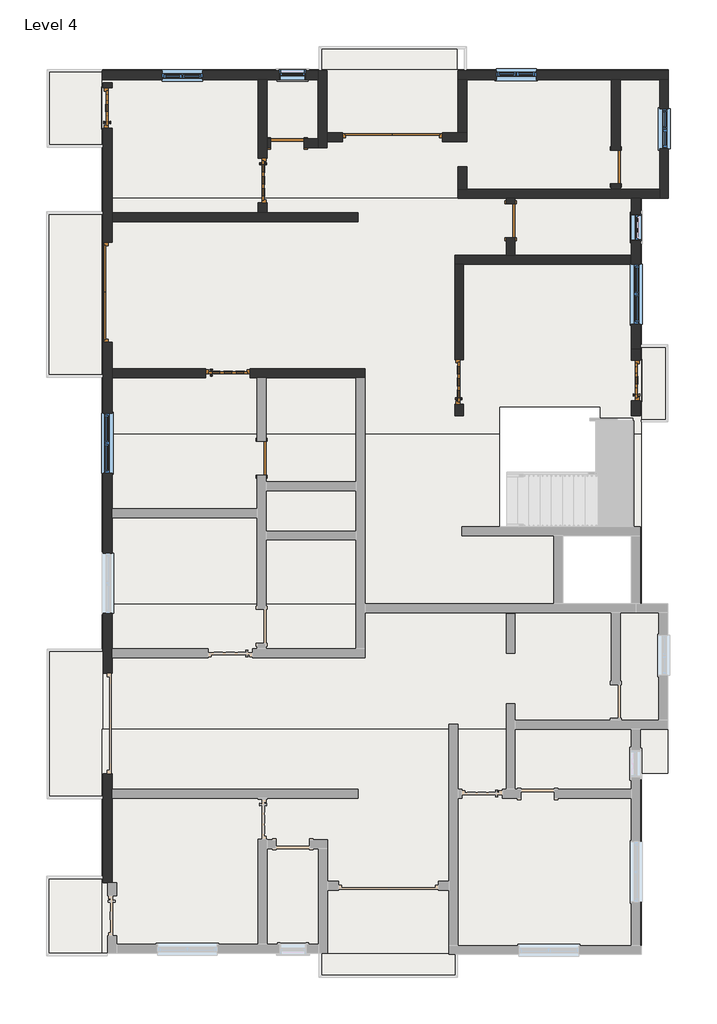
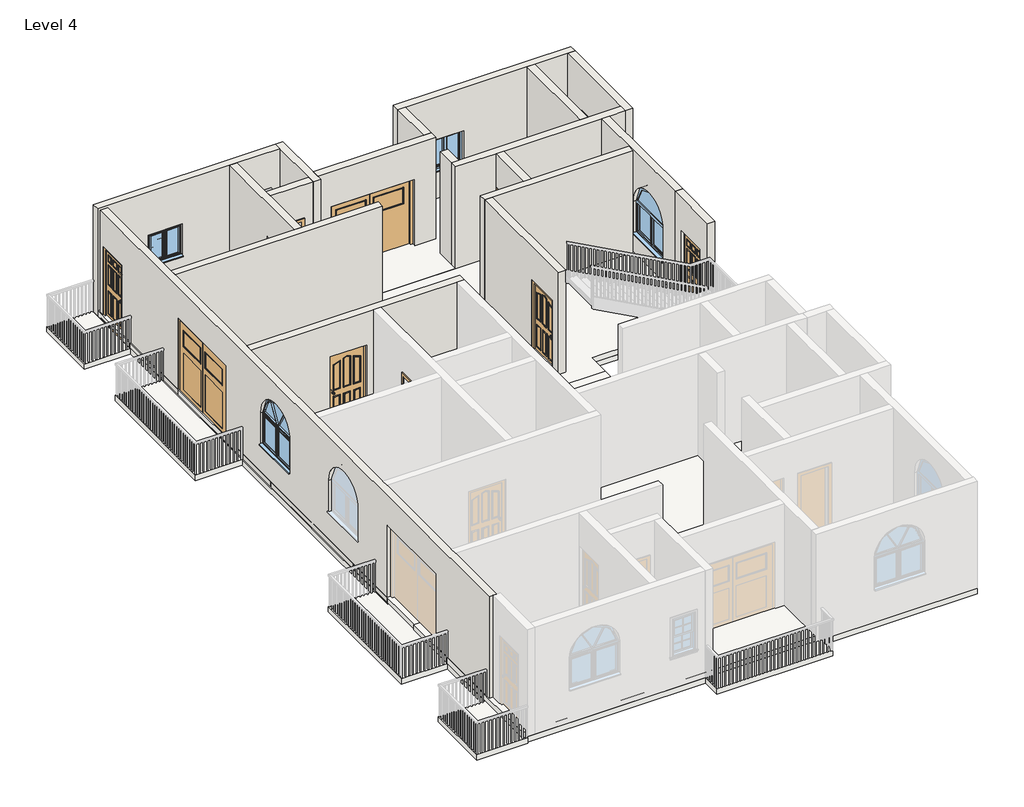
# One storey, part 2 of 7: 19 walls, 11 doors, 10 slabs, 7 windows, 5 roofs.
"""IFC4 building model written with IfcOpenShell, lengths in millimetres."""

from ifc_helpers import new_model, si_unit, point, frame, frame_2d, origin, place, context, project, spatial, polyline, circle_curve, trimmed, segment, composite_curve, outline, extrude, faceted_brep, transform, mapped, element, save
from ifc_brep_helpers import plane_surface, revolved_surface, advanced_brep
from components import doors_extsgl_5_910x2110mm_99758a98, doors_extsgl_5_910x2110mm_d3ca6061, doors_extsgl_6_1010x2110mm_b93c615f, doors_extsgl_6_1010x2110mm_efbaf1af, doors_garage_timber_side_hung_glazing_2270x2050mm_ae99176d, doors_garage_timber_side_hung_glazing_2270x2200mm_badb7014, door_53b1b562, window_679d2811, windows_arched_1360x910mm_c5754810, windows_dbl_w_glazing_bars_910x910mm_41eba874

model = new_model("IFC4")

# Units and contexts
model_context = context("Model", 3, world=origin())
ifc_project = project(units=[si_unit("LENGTHUNIT", "METRE", prefix="MILLI")], contexts=[model_context])

# Site, building, storey
site = spatial("IfcSite", under=ifc_project)
building = spatial("IfcBuilding", under=site)
storey = spatial("IfcBuildingStorey", under=building, Name="Level 4", Elevation=9144.0)

# Doors
placement = place(None, origin())
doors_extsgl_5_910x2110mm_shape = doors_extsgl_5_910x2110mm_99758a98(model_context)
element("IfcDoor", 1, ObjectType="Doors_ExtSgl_5 : 910x2110mm", at=placement, inside=storey, context=model_context, shape_type="MappedRepresentation", body=[
    mapped(doors_extsgl_5_910x2110mm_shape, transform((5761.5890963, 2376.5107951, 9144.0), x_axis=(0.0, 1.0, 0.0), y_axis=(-1.0, 0.0, 0.0), z_axis=(0.0, 0.0, 1.0))),
])
doors_extsgl_5_910x2110mm_2_shape = doors_extsgl_5_910x2110mm_d3ca6061(model_context)
element("IfcDoor", 2, ObjectType="Doors_ExtSgl_5 : 910x2110mm", at=placement, inside=storey, context=model_context, shape_type="MappedRepresentation", body=[
    mapped(doors_extsgl_5_910x2110mm_2_shape, transform((-6229.2013636, 8553.74399, 9144.0), x_axis=(0.0, 1.0, 0.0), y_axis=(-1.0, 0.0, 0.0), z_axis=(0.0, 0.0, 1.0))),
])
doors_extsgl_6_1010x2110mm_shape = doors_extsgl_6_1010x2110mm_b93c615f(model_context)
doors_extsgl_6_1010x2110mm_2_shape = doors_extsgl_6_1010x2110mm_efbaf1af(model_context)
element("IfcDoor", 3, ObjectType="Doors_ExtSgl_6 : 1010x2110mm", at=placement, inside=storey, context=model_context, shape_type="MappedRepresentation", body=[
    mapped(doors_extsgl_6_1010x2110mm_shape, transform((-2709.3109037, 6913.1295584, 9144.0), x_axis=(0.0, -1.0, 0.0), y_axis=(1.0, 0.0, 0.0), z_axis=(0.0, 0.0, 1.0))),
    mapped(doors_extsgl_6_1010x2110mm_2_shape, transform((-2709.3109037, 6913.1295584, 9144.0), x_axis=(0.0, -1.0, 0.0), y_axis=(1.0, 0.0, 0.0), z_axis=(0.0, 0.0, 1.0))),
])
element("IfcDoor", 4, ObjectType="Doors_ExtSgl_6 : 1010x2110mm", at=placement, inside=storey, context=model_context, shape_type="MappedRepresentation", body=[
    mapped(doors_extsgl_6_1010x2110mm_shape, transform((1748.3890963, 2341.0628918, 9144.0), x_axis=(0.0, 1.0, 0.0), y_axis=(-1.0, 0.0, 0.0), z_axis=(0.0, 0.0, 1.0))),
    mapped(doors_extsgl_6_1010x2110mm_2_shape, transform((1748.3890963, 2341.0628918, 9144.0), x_axis=(0.0, 1.0, 0.0), y_axis=(-1.0, 0.0, 0.0), z_axis=(0.0, 0.0, 1.0))),
])
element("IfcDoor", 5, ObjectType="Doors_ExtSgl_6 : 1010x2110mm", at=placement, inside=storey, context=model_context, shape_type="MappedRepresentation", body=[
    mapped(doors_extsgl_6_1010x2110mm_shape, transform((-3496.7442371, 2544.2962251, 9144.0), x_axis=(1.0, 0.0, 0.0), y_axis=(0.0, 1.0, 0.0), z_axis=(0.0, 0.0, 1.0))),
    mapped(doors_extsgl_6_1010x2110mm_2_shape, transform((-3496.7442371, 2544.2962251, 9144.0), x_axis=(1.0, 0.0, 0.0), y_axis=(0.0, 1.0, 0.0), z_axis=(0.0, 0.0, 1.0))),
])
doors_garage_timber_side_hung_glazing_2270x2050mm_shape = doors_garage_timber_side_hung_glazing_2270x2050mm_ae99176d(model_context)
element("IfcDoor", 6, ObjectType="Doors_Garage_Timber_Side_Hung_Glazing : 2270x2050mm", at=placement, inside=storey, context=model_context, shape_type="MappedRepresentation", body=[
    mapped(doors_garage_timber_side_hung_glazing_2270x2050mm_shape, transform((237.0890963, 7890.9962251, 9144.0), x_axis=(1.0, 0.0, 0.0), y_axis=(0.0, 1.0, 0.0), z_axis=(0.0, 0.0, 1.0))),
])
doors_garage_timber_side_hung_glazing_2270x2200mm_shape = doors_garage_timber_side_hung_glazing_2270x2200mm_badb7014(model_context)
element("IfcDoor", 7, ObjectType="Doors_Garage_Timber_Side_Hung_Glazing : 2270x2200mm", at=placement, inside=storey, context=model_context, shape_type="MappedRepresentation", body=[
    mapped(doors_garage_timber_side_hung_glazing_2270x2200mm_shape, transform((-6229.2013636, 4373.0962251, 9144.0), x_axis=(0.0, -1.0, 0.0), y_axis=(1.0, 0.0, 0.0), z_axis=(0.0, 0.0, 1.0))),
])
door_shape = door_53b1b562(model_context)
element("IfcDoor", 8, ObjectType="Single-Flush : 30\" x 80\"", at=placement, inside=storey, context=model_context, shape_type="MappedRepresentation", body=[
    mapped(door_shape, transform((-2150.5109037, 7751.2962251, 9144.0), x_axis=(-1.0, 0.0, 0.0), y_axis=(0.0, -1.0, 0.0), z_axis=(0.0, 0.0, 1.0))),
])
element("IfcDoor", 9, ObjectType="Single-Flush : 30\" x 80\"", at=placement, inside=storey, context=model_context, shape_type="MappedRepresentation", body=[
    mapped(door_shape, transform((2916.7890963, 5998.6962251, 9144.0), x_axis=(0.0, 1.0, 0.0), y_axis=(-1.0, 0.0, 0.0), z_axis=(0.0, 0.0, 1.0))),
])
element("IfcDoor", 10, ObjectType="Single-Flush : 30\" x 80\"", at=placement, inside=storey, context=model_context, shape_type="MappedRepresentation", body=[
    mapped(door_shape, transform((-2734.7109037, 613.8962251, 9144.0), x_axis=(0.0, 1.0, 0.0), y_axis=(-1.0, 0.0, 0.0), z_axis=(0.0, 0.0, 1.0))),
])
element("IfcDoor", 11, ObjectType="Single-Flush : 30\" x 80\"", at=placement, inside=storey, context=model_context, shape_type="MappedRepresentation", body=[
    mapped(door_shape, transform((5304.3890963, 7217.8962251, 9144.0), x_axis=(0.0, 1.0, 0.0), y_axis=(-1.0, 0.0, 0.0), z_axis=(0.0, 0.0, 1.0))),
])

# Roofs
element("IfcRoof", 12, ObjectType="Generic - 12\"", at=placement, inside=storey, context=model_context, shape_type="SweptSolid", body=[
    extrude(outline(polyline([(-6354.2109037, 9427.2527313), (6498.1890963, 9427.2527313), (6498.1890963, 6506.6962251), (-6354.2109037, 6506.6962251), (-6354.2109037, 9427.2527313)])), frame((0.0, 0.0, 9144.0), z_axis=(0.0, 0.0, 1.0), x_axis=(1.0, 0.0, 0.0)), (0.0, 0.0, 1.0), 152.4),
])
element("IfcRoof", 13, ObjectType="Generic - 12\"", at=placement, inside=storey, context=model_context, shape_type="SweptSolid", body=[
    extrude(outline(polyline([(-6330.8013636, -2688.1037749), (6485.4890963, -2688.1037749), (6485.4890963, -6529.1251987), (-6330.8013636, -6529.1251987), (-6330.8013636, -2688.1037749)])), frame((0.0, 0.0, 9144.0), z_axis=(0.0, 0.0, 1.0), x_axis=(1.0, 0.0, 0.0)), (0.0, 0.0, 1.0), 152.4),
])
element("IfcRoof", 14, ObjectType="Generic - 12\"", at=placement, inside=storey, context=model_context, shape_type="SweptSolid", body=[
    extrude(outline(polyline([(-6354.2109037, -5532.9037749), (5863.1890963, -5532.9037749), (5863.1890963, -10612.9037749), (-6354.2109037, -10612.9037749), (-6354.2109037, -5532.9037749)])), frame((0.0, 0.0, 9144.0), z_axis=(0.0, 0.0, 1.0), x_axis=(1.0, 0.0, 0.0)), (0.0, 0.0, 1.0), 152.4),
])
element("IfcRoof", 15, ObjectType="Generic - 12\"", at=placement, inside=storey, context=model_context, shape_type="SweptSolid", body=[
    extrude(outline(polyline([(-6330.8013636, 1160.801054), (-6330.8013636, 6506.6962251), (5875.8890963, 6506.6962251), (5875.8890963, 1160.801054), (4949.8616623, 1160.801054), (4949.8616623, 1784.6684315), (2663.8616623, 1784.6684315), (2663.8616623, 1160.801054), (-6330.8013636, 1160.801054)])), frame((0.0, 0.0, 9144.0), z_axis=(0.0, 0.0, 1.0), x_axis=(1.0, 0.0, 0.0)), (0.0, 0.0, 1.0), 152.4),
])
element("IfcRoof", 16, ObjectType="Generic - 12\"", at=placement, inside=storey, context=model_context, shape_type="SweptSolid", body=[
    extrude(outline(polyline([(-6330.8013636, -2688.1037749), (-6330.8013636, 1160.801054), (2663.8616623, 1160.801054), (2663.8616623, -958.5315685), (4949.8616623, -958.5315685), (4949.8616623, 1160.801054), (5875.8890963, 1160.801054), (5875.8890963, -2688.1037749), (5659.9890963, -2688.1037749), (5659.9890963, -1138.7037749), (4097.8890963, -1138.7037749), (4097.8890963, -2688.1037749), (-6330.8013636, -2688.1037749)])), frame((0.0, 0.0, 9144.0), z_axis=(0.0, 0.0, 1.0), x_axis=(1.0, 0.0, 0.0)), (0.0, 0.0, 1.0), 152.4),
])

# Slabs
element("IfcSlab", 17, ObjectType="Generic - 12\"", at=placement, inside=storey, context=model_context, shape_type="SweptSolid", body=[
    extrude(outline(polyline([(1694.4140963, 9948.3962251), (1694.4140963, -11133.6037749), (-1426.6109037, -11133.6037749), (-1426.6109037, 9948.3962251), (1694.4140963, 9948.3962251)])), frame((0.0, 0.0, 8991.6), z_axis=(0.0, 0.0, 1.0), x_axis=(1.0, 0.0, 0.0)), (0.0, 0.0, 1.0), 152.4),
])
element("IfcSlab", 18, ObjectType="Generic - 12\"", at=placement, inside=storey, context=model_context, shape_type="SweptSolid", body=[
    extrude(outline(polyline([(5875.8890963, 9402.2962251), (5875.8890963, -10638.3037749), (1722.9890963, -10638.3037749), (1722.9890963, 9402.2962251), (5875.8890963, 9402.2962251)]), holes=[polyline([(4949.8616623, 1784.6684315), (2663.8616623, 1784.6684315), (2663.8616623, -958.5315685), (4949.8616623, -958.5315685), (4949.8616623, 1784.6684315)]), polyline([(5659.9890963, -1138.7037749), (4097.8890963, -1138.7037749), (4097.8890963, -2688.1037749), (5659.9890963, -2688.1037749), (5659.9890963, -1138.7037749)])]), frame((0.0, 0.0, 8991.6), z_axis=(0.0, 0.0, 1.0), x_axis=(1.0, 0.0, 0.0)), (0.0, 0.0, 1.0), 152.4),
])
element("IfcSlab", 19, ObjectType="Generic - 12\"", at=placement, inside=storey, context=model_context, shape_type="SweptSolid", body=[
    extrude(outline(polyline([(6498.1890963, 9402.2962251), (6498.1890963, 6506.6962251), (5875.8890963, 6506.6962251), (5875.8890963, 9402.2962251), (6498.1890963, 9402.2962251)])), frame((0.0, 0.0, 8991.6), z_axis=(0.0, 0.0, 1.0), x_axis=(1.0, 0.0, 0.0)), (0.0, 0.0, 1.0), 152.4),
])
element("IfcSlab", 20, ObjectType="Generic - 12\"", at=placement, inside=storey, context=model_context, shape_type="SweptSolid", body=[
    extrude(outline(polyline([(6485.4890963, 3183.81308), (6485.4890963, 1439.3962251), (5863.1890963, 1439.3962251), (5863.1890963, 3183.81308), (6485.4890963, 3183.81308)])), frame((0.0, 0.0, 8991.6), z_axis=(0.0, 0.0, 1.0), x_axis=(1.0, 0.0, 0.0)), (0.0, 0.0, 1.0), 152.4),
])
element("IfcSlab", 21, ObjectType="Generic - 12\"", at=placement, inside=storey, context=model_context, shape_type="SweptSolid", body=[
    extrude(outline(polyline([(6485.4890963, -2688.1037749), (6485.4890963, -5532.9037749), (5863.1890963, -5532.9037749), (5863.1890963, -2688.1037749), (6485.4890963, -2688.1037749)])), frame((0.0, 0.0, 8991.6), z_axis=(0.0, 0.0, 1.0), x_axis=(1.0, 0.0, 0.0)), (0.0, 0.0, 1.0), 152.4),
])
element("IfcSlab", 22, ObjectType="Generic - 12\"", at=placement, inside=storey, context=model_context, shape_type="SweptSolid", body=[
    extrude(outline(polyline([(-6330.8013636, 9427.2527313), (-6330.8013636, 7667.1584215), (-7598.8109037, 7667.1584215), (-7598.8109037, 9427.2527313), (-6330.8013636, 9427.2527313)])), frame((0.0, 0.0, 8991.6), z_axis=(0.0, 0.0, 1.0), x_axis=(1.0, 0.0, 0.0)), (0.0, 0.0, 1.0), 152.4),
])
element("IfcSlab", 23, ObjectType="Generic - 12\"", at=placement, inside=storey, context=model_context, shape_type="SweptSolid", body=[
    extrude(outline(polyline([(-6330.8013636, 6201.8962251), (-6330.8013636, 2455.3962251), (-7614.6859037, 2455.3962251), (-7614.6859037, 6201.8962251), (-6330.8013636, 6201.8962251)])), frame((0.0, 0.0, 8991.6), z_axis=(0.0, 0.0, 1.0), x_axis=(1.0, 0.0, 0.0)), (0.0, 0.0, 1.0), 152.4),
])
element("IfcSlab", 24, ObjectType="Generic - 12\"", at=placement, inside=storey, context=model_context, shape_type="SweptSolid", body=[
    extrude(outline(polyline([(-6330.8013636, -3716.8037749), (-6330.8013636, -7105.2894702), (-7598.8109037, -7105.2894702), (-7598.8109037, -3716.8037749), (-6330.8013636, -3716.8037749)])), frame((0.0, 0.0, 8991.6), z_axis=(0.0, 0.0, 1.0), x_axis=(1.0, 0.0, 0.0)), (0.0, 0.0, 1.0), 152.4),
])
element("IfcSlab", 25, ObjectType="Generic - 12\"", at=placement, inside=storey, context=model_context, shape_type="SweptSolid", body=[
    extrude(outline(polyline([(-6243.0859037, -8868.0845215), (-6243.0859037, -10663.7037749), (-7614.6859037, -10663.7037749), (-7614.6859037, -8868.0845215), (-6243.0859037, -8868.0845215)])), frame((0.0, 0.0, 8991.6), z_axis=(0.0, 0.0, 1.0), x_axis=(1.0, 0.0, 0.0)), (0.0, 0.0, 1.0), 152.4),
])
element("IfcSlab", 26, ObjectType="Generic - 12\"", at=placement, inside=storey, context=model_context, shape_type="SweptSolid", body=[
    extrude(outline(polyline([(-1236.1109037, 9427.2527313), (-1236.1109037, -10612.9037749), (-6354.2109037, -10612.9037749), (-6354.2109037, 9427.2527313), (-1236.1109037, 9427.2527313)])), frame((0.0, 0.0, 8991.6), z_axis=(0.0, 0.0, 1.0), x_axis=(1.0, 0.0, 0.0)), (0.0, 0.0, 1.0), 152.4),
])

# Walls
element("IfcWall", 27, ObjectType="Generic - 9\" w", at=placement, inside=storey, context=model_context, shape_type="Brep", body=[
    faceted_brep([(1722.9890963, 9199.0962251, 9144.0), (1926.1890963, 9199.0962251, 9144.0), (5202.7890963, 9199.0962251, 9144.0), (5405.9890963, 9199.0962251, 9144.0), (6294.9890963, 9199.0962251, 9144.0), (6498.1890963, 9199.0962251, 9144.0), (6498.1890963, 9199.0962251, 12192.0), (6294.9890963, 9199.0962251, 12192.0), (5405.9890963, 9199.0962251, 12192.0), (5202.7890963, 9199.0962251, 12192.0), (1926.1890963, 9199.0962251, 12192.0), (1722.9890963, 9199.0962251, 12192.0), (2588.7890963, 9199.0962251, 10968.4), (3498.7890963, 9199.0962251, 10968.4), (3498.7890963, 9199.0962251, 10058.4), (2588.7890963, 9199.0962251, 10058.4), (1722.9890963, 9402.2962251, 9144.0), (1722.9890963, 9402.2962251, 12192.0), (6498.1890963, 9402.2962251, 12192.0), (6498.1890963, 9402.2962251, 9144.0), (2588.7890963, 9402.2962251, 10968.4), (2588.7890963, 9402.2962251, 10058.4), (3498.7890963, 9402.2962251, 10058.4), (3498.7890963, 9402.2962251, 10968.4)], [[[0, 1, 2, 3, 4, 5, 6, 7, 8, 9, 10, 11], [12, 13, 14, 15]], [[16, 17, 18, 19], [20, 21, 22, 23]], [[5, 4, 3, 2, 1, 0, 16, 19]], [[11, 10, 9, 8, 7, 6, 18, 17]], [[0, 11, 17, 16]], [[6, 5, 19, 18]], [[21, 20, 12, 15]], [[22, 21, 15, 14]], [[23, 22, 14, 13]], [[20, 23, 13, 12]]]),
])
element("IfcWall", 28, ObjectType="Generic - 9\" w", at=placement, inside=storey, context=model_context, shape_type="SweptSolid", body=[
    extrude(outline(polyline([(6506.6962251, 9144.0), (3087.7441284, 9144.0), (3087.7441284, 12192.0), (6506.6962251, 12192.0), (6506.6962251, 9144.0)]), holes=[polyline([(6151.0962251, 11125.2), (5541.4962251, 11125.2), (5541.4962251, 10058.4), (6151.0962251, 10058.4), (6151.0962251, 11125.2)]), composite_curve([segment(polyline([(5016.7786331, 9829.6617803), (5016.7786331, 10739.6617803)]), True, "CONTINUOUS"), segment(trimmed(circle_curve(frame_2d((4336.7786331, 10739.6617803)), 680.0), [point((5016.7786331, 10739.6617803))], [point((3656.7786331, 10739.6617803))], True, "CARTESIAN"), True, "CONTINUOUS"), segment(polyline([(3656.7786331, 10739.6617803), (3656.7786331, 9829.6617803), (5016.7786331, 9829.6617803)]), True, "CONTINUOUS")], self_intersect=False)]), frame((5659.9890963, 0.0, 0.0), z_axis=(1.0, 0.0, 0.0), x_axis=(0.0, 1.0, 0.0)), (0.0, 0.0, 1.0), 203.2),
])
element("IfcWall", 29, ObjectType="Generic - 9\" w", at=placement, inside=storey, context=model_context, shape_type="AdvancedBrep", body=[
    advanced_brep(
    [(-6330.8013636, 3238.0962251, 9144.0), (-6330.8013636, -4267.1251987, 9144.0), (-6330.8013636, -4267.1251987, 11344.0), (-6330.8013636, -6537.1251987, 11344.0), (-6330.8013636, -6537.1251987, 9144.0), (-6330.8013636, -9007.7845215, 9144.0), (-6330.8013636, -9007.7845215, 12192.0), (-6330.8013636, 9129.8816143, 12192.0), (-6330.8013636, 9129.8816143, 9144.0), (-6330.8013636, 9008.7773233, 9144.0), (-6330.8013636, 9008.7773233, 11254.0), (-6330.8013636, 8098.7773233, 11254.0), (-6330.8013636, 8098.7773233, 9144.0), (-6330.8013636, 5508.0962251, 9144.0), (-6330.8013636, 5508.0962251, 11344.0), (-6330.8013636, 3238.0962251, 11344.0), (-6330.8013636, 276.7962251, 10058.4), (-6330.8013636, 1636.7962251, 10058.4), (-6330.8013636, 1636.7962251, 10968.4), (-6330.8013636, 276.7962251, 10968.4), (-6330.8013636, -1538.2037749, 10058.4), (-6330.8013636, -1538.2037749, 10968.4), (-6330.8013636, -2898.2037749, 10968.4), (-6330.8013636, -2898.2037749, 10058.4), (-6127.6013636, -4267.1251987, 11344.0), (-6127.6013636, -4267.1251987, 9144.0), (-6127.6013636, -3907.3037749, 9144.0), (-6127.6013636, -3704.1037749, 9144.0), (-6127.6013636, -732.3037749, 9144.0), (-6127.6013636, -529.1037749, 9144.0), (-6127.6013636, 2442.6962251, 9144.0), (-6127.6013636, 2645.8962251, 9144.0), (-6127.6013636, 3238.0962251, 9144.0), (-6127.6013636, 3238.0962251, 11344.0), (-6127.6013636, 5508.0962251, 11344.0), (-6127.6013636, 5508.0962251, 9144.0), (-6127.6013636, 5973.2962251, 9144.0), (-6127.6013636, 6176.4962251, 9144.0), (-6127.6013636, 8098.7773233, 9144.0), (-6127.6013636, 8098.7773233, 11254.0), (-6127.6013636, 9008.7773233, 11254.0), (-6127.6013636, 9008.7773233, 9144.0), (-6127.6013636, 9129.8816143, 9144.0), (-6127.6013636, 9129.8816143, 12192.0), (-6127.6013636, 6176.4962251, 12192.0), (-6127.6013636, 5973.2962251, 12192.0), (-6127.6013636, 2645.8962251, 12192.0), (-6127.6013636, 2442.6962251, 12192.0), (-6127.6013636, -529.1037749, 12192.0), (-6127.6013636, -732.3037749, 12192.0), (-6127.6013636, -3704.1037749, 12192.0), (-6127.6013636, -3907.3037749, 12192.0), (-6127.6013636, -6896.9466225, 12192.0), (-6127.6013636, -7100.1466225, 12192.0), (-6127.6013636, -9007.7845215, 12192.0), (-6127.6013636, -9007.7845215, 9144.0), (-6127.6013636, -7100.1466225, 9144.0), (-6127.6013636, -6896.9466225, 9144.0), (-6127.6013636, -6537.1251987, 9144.0), (-6127.6013636, -6537.1251987, 11344.0), (-6127.6013636, 276.7962251, 10058.4), (-6127.6013636, 276.7962251, 10968.4), (-6127.6013636, 1636.7962251, 10968.4), (-6127.6013636, 1636.7962251, 10058.4), (-6127.6013636, -1538.2037749, 10058.4), (-6127.6013636, -2898.2037749, 10058.4), (-6127.6013636, -2898.2037749, 10968.4), (-6127.6013636, -1538.2037749, 10968.4), (-6229.2013636, -9007.7845215, 9144.0), (-6229.2013636, -9007.7845215, 12192.0)],
    [
        (0, 1),
        (1, 2),
        (2, 3),
        (3, 4),
        (4, 5),
        (5, 6),
        (6, 7),
        (7, 8),
        (8, 9),
        (9, 10),
        (10, 11),
        (11, 12),
        (12, 13),
        (13, 14),
        (14, 15),
        (15, 0),
        (16, 17),
        (17, 18),
        (18, 19, circle_curve(frame((-6330.8013636, 956.7962251, 10968.4), z_axis=(1.0, 0.0, 0.0), x_axis=(0.0, 1.0, 0.0)), 680.0)),
        (19, 16),
        (20, 21),
        (21, 22, circle_curve(frame((-6330.8013636, -2218.2037749, 10968.4), z_axis=(1.0, 0.0, 0.0), x_axis=(0.0, -1.0, 0.0)), 680.0)),
        (22, 23),
        (23, 20),
        (24, 25),
        (25, 26),
        (26, 27),
        (27, 28),
        (28, 29),
        (29, 30),
        (30, 31),
        (31, 32),
        (32, 33),
        (33, 34),
        (34, 35),
        (35, 36),
        (36, 37),
        (37, 38),
        (38, 39),
        (39, 40),
        (40, 41),
        (41, 42),
        (42, 43),
        (43, 44),
        (44, 45),
        (45, 46),
        (46, 47),
        (47, 48),
        (48, 49),
        (49, 50),
        (50, 51),
        (51, 52),
        (52, 53),
        (53, 54),
        (54, 55),
        (55, 56),
        (56, 57),
        (57, 58),
        (58, 59),
        (59, 24),
        (60, 61),
        (61, 62, circle_curve(frame((-6127.6013636, 956.7962251, 10968.4), z_axis=(-1.0, 0.0, 0.0), x_axis=(0.0, 1.0, 0.0)), 680.0)),
        (62, 63),
        (63, 60),
        (64, 65),
        (65, 66),
        (66, 67, circle_curve(frame((-6127.6013636, -2218.2037749, 10968.4), z_axis=(-1.0, 0.0, 0.0), x_axis=(0.0, -1.0, 0.0)), 680.0)),
        (67, 64),
        (41, 9),
        (8, 42),
        (12, 38),
        (35, 13),
        (55, 68),
        (68, 5),
        (4, 58),
        (25, 1),
        (0, 32),
        (54, 69),
        (69, 6),
        (43, 7),
        (11, 39),
        (40, 10),
        (34, 14),
        (15, 33),
        (3, 59),
        (24, 2),
        (60, 16),
        (19, 61),
        (18, 62),
        (17, 63),
        (20, 64),
        (67, 21),
        (66, 22),
        (65, 23),
    ],
    [
        plane_surface(frame((-6330.8013636, 2442.6962251, 9144.0), z_axis=(-1.0, 0.0, 0.0), x_axis=(0.0, -1.0, 0.0))),
        plane_surface(frame((-6127.6013636, 2442.6962251, 9144.0), z_axis=(1.0, 0.0, 0.0), x_axis=(0.0, 1.0, 0.0))),
        plane_surface(frame((-6330.8013636, 9129.8816143, 9144.0), z_axis=(0.0, 0.0, -1.0), x_axis=(1.0, 0.0, 0.0))),
        plane_surface(frame((-6330.8013636, -9007.7845215, 9144.0), z_axis=(0.0, -1.0, 0.0), x_axis=(1.0, 0.0, 0.0))),
        plane_surface(frame((-6330.8013636, -9007.7845215, 12192.0), z_axis=(0.0, 0.0, 1.0), x_axis=(1.0, 0.0, 0.0))),
        plane_surface(frame((-6330.8013636, 9129.8816143, 12192.0), z_axis=(0.0, 1.0, 0.0), x_axis=(1.0, 0.0, 0.0))),
        plane_surface(frame((-6330.8013636, 8098.7773233, 11254.0), z_axis=(0.0, 1.0, 0.0), x_axis=(1.0, 0.0, 0.0))),
        plane_surface(frame((-6330.8013636, 9008.7773233, 9144.0), z_axis=(0.0, -1.0, 0.0), x_axis=(1.0, 0.0, 0.0))),
        plane_surface(frame((-6330.8013636, 9008.7773233, 11254.0), z_axis=(0.0, 0.0, -1.0), x_axis=(1.0, 0.0, 0.0))),
        plane_surface(frame((-6127.6013636, 5508.0962251, 11344.0), z_axis=(0.0, -1.0, 0.0), x_axis=(-1.0, 0.0, 0.0))),
        plane_surface(frame((-6127.6013636, 3238.0962251, 9144.0), z_axis=(0.0, 1.0, 0.0), x_axis=(-1.0, 0.0, 0.0))),
        plane_surface(frame((-6127.6013636, 3238.0962251, 11344.0), z_axis=(0.0, 0.0, -1.0), x_axis=(-1.0, 0.0, 0.0))),
        plane_surface(frame((-6330.8013636, -6537.1251987, 11344.0), z_axis=(0.0, 1.0, 0.0), x_axis=(1.0, 0.0, 0.0))),
        plane_surface(frame((-6330.8013636, -4267.1251987, 9144.0), z_axis=(0.0, -1.0, 0.0), x_axis=(1.0, 0.0, 0.0))),
        plane_surface(frame((-6330.8013636, -4267.1251987, 11344.0), z_axis=(0.0, 0.0, -1.0), x_axis=(1.0, 0.0, 0.0))),
        plane_surface(frame((-6127.6013636, 276.7962251, 10058.4), z_axis=(0.0, 1.0, 0.0), x_axis=(-1.0, 0.0, 0.0))),
        revolved_surface(polyline([(-6330.8013636, 1636.7962251, 10968.4), (-6127.6013636, 1636.7962251, 10968.4)]), (-6127.6013636, 956.7962251, 10968.4), (-1.0, 0.0, 0.0)),
        plane_surface(frame((-6127.6013636, 1636.7962251, 10968.4), z_axis=(0.0, -1.0, 0.0), x_axis=(-1.0, 0.0, 0.0))),
        plane_surface(frame((-6127.6013636, 1636.7962251, 10058.4), z_axis=(0.0, 0.0, 1.0), x_axis=(-1.0, 0.0, 0.0))),
        plane_surface(frame((-6330.8013636, -1538.2037749, 10058.4), z_axis=(0.0, -1.0, 0.0), x_axis=(1.0, 0.0, 0.0))),
        revolved_surface(polyline([(-6127.6013636, -2898.2037749, 10968.4), (-6330.8013636, -2898.2037749, 10968.4)]), (-6330.8013636, -2218.2037749, 10968.4), (1.0, 0.0, 0.0)),
        plane_surface(frame((-6330.8013636, -2898.2037749, 10968.4), z_axis=(0.0, 1.0, 0.0), x_axis=(1.0, 0.0, 0.0))),
        plane_surface(frame((-6330.8013636, -2898.2037749, 10058.4), z_axis=(0.0, 0.0, 1.0), x_axis=(1.0, 0.0, 0.0))),
    ],
    [
        (0, [[1, 2, 3, 4, 5, 6, 7, 8, 9, 10, 11, 12, 13, 14, 15, 16], [17, 18, 19, 20], [21, 22, 23, 24]]),
        (1, [[25, 26, 27, 28, 29, 30, 31, 32, 33, 34, 35, 36, 37, 38, 39, 40, 41, 42, 43, 44, 45, 46, 47, 48, 49, 50, 51, 52, 53, 54, 55, 56, 57, 58, 59, 60], [61, 62, 63, 64], [65, 66, 67, 68]]),
        (2, [[-42, 69, -9, 70]]),
        (2, [[-13, 71, -38, -37, -36, 72]]),
        (2, [[-58, -57, -56, 73, 74, -5, 75]]),
        (2, [[-32, -31, -30, -29, -28, -27, -26, 76, -1, 77]]),
        (3, [[-6, -74, -73, -55, 78, 79]]),
        (4, [[-7, -79, -78, -54, -53, -52, -51, -50, -49, -48, -47, -46, -45, -44, 80]]),
        (5, [[-8, -80, -43, -70]]),
        (6, [[-12, 81, -39, -71]]),
        (7, [[-10, -69, -41, 82]]),
        (8, [[-11, -82, -40, -81]]),
        (9, [[-35, 83, -14, -72]]),
        (10, [[-33, -77, -16, 84]]),
        (11, [[-34, -84, -15, -83]]),
        (12, [[-4, 85, -59, -75]]),
        (13, [[-2, -76, -25, 86]]),
        (14, [[-3, -86, -60, -85]]),
        (15, [[-61, 87, -20, 88]]),
        (16, [[-62, -88, -19, 89]]),
        (17, [[-63, -89, -18, 90]]),
        (18, [[-64, -90, -17, -87]]),
        (19, [[-21, 91, -68, 92]]),
        (20, [[-22, -92, -67, 93]]),
        (21, [[-23, -93, -66, 94]]),
        (22, [[-24, -94, -65, -91]]),
    ],
),
])
element("IfcWall", 30, ObjectType="Generic - 9\" w", at=placement, inside=storey, context=model_context, shape_type="SweptSolid", body=[
    extrude(outline(polyline([(3087.7441284, 9144.0), (2831.5441284, 9144.0), (2831.5441284, 11254.0), (1921.5441284, 11254.0), (1921.5441284, 9144.0), (1579.0962251, 9144.0), (1579.0962251, 12192.0), (3087.7441284, 12192.0), (3087.7441284, 9144.0)])), frame((5659.9890963, 0.0, 0.0), z_axis=(1.0, 0.0, 0.0), x_axis=(0.0, 1.0, 0.0)), (0.0, 0.0, 1.0), 203.2),
])
element("IfcWall", 31, ObjectType="Generic - 9\" w", at=placement, inside=storey, context=model_context, shape_type="Brep", body=[
    faceted_brep([(-1452.0109037, 9401.8527313, 9144.0), (-6354.2109037, 9401.8527313, 9144.0), (-6354.2109037, 9401.8527313, 12192.0), (-1452.0109037, 9401.8527313, 12192.0), (-4076.7609037, 9401.8527313, 10968.4), (-4986.7609037, 9401.8527313, 10968.4), (-4986.7609037, 9401.8527313, 10058.4), (-4076.7609037, 9401.8527313, 10058.4), (-2334.6609037, 9401.8527313, 11125.2), (-2334.6609037, 9401.8527313, 10058.4), (-1725.0609037, 9401.8527313, 10058.4), (-1725.0609037, 9401.8527313, 11125.2), (-1452.0109037, 9198.6527313, 9144.0), (-1452.0109037, 9198.6527313, 12192.0), (-2607.7109037, 9198.6527313, 12192.0), (-2810.9109037, 9198.6527313, 12192.0), (-6354.2109037, 9198.6527313, 12192.0), (-6354.2109037, 9198.6527313, 9144.0), (-2810.9109037, 9198.6527313, 9144.0), (-2607.7109037, 9198.6527313, 9144.0), (-4076.7609037, 9198.6527313, 10968.4), (-4076.7609037, 9198.6527313, 10058.4), (-4986.7609037, 9198.6527313, 10058.4), (-4986.7609037, 9198.6527313, 10968.4), (-2334.6609037, 9198.6527313, 11125.2), (-1725.0609037, 9198.6527313, 11125.2), (-1725.0609037, 9198.6527313, 10058.4), (-2334.6609037, 9198.6527313, 10058.4)], [[[0, 1, 2, 3], [4, 5, 6, 7], [8, 9, 10, 11]], [[12, 13, 14, 15, 16, 17, 18, 19], [20, 21, 22, 23], [24, 25, 26, 27]], [[1, 0, 12, 19, 18, 17]], [[2, 1, 17, 16]], [[3, 2, 16, 15, 14, 13]], [[0, 3, 13, 12]], [[21, 20, 4, 7]], [[22, 21, 7, 6]], [[23, 22, 6, 5]], [[20, 23, 5, 4]], [[9, 8, 24, 27]], [[10, 9, 27, 26]], [[11, 10, 26, 25]], [[8, 11, 25, 24]]]),
])
element("IfcWall", 32, ObjectType="Generic -4.5\" p", at=placement, inside=storey, context=model_context, shape_type="Brep", body=[
    faceted_brep([(-2810.9109037, 6408.0962251, 11254.0), (-2810.9109037, 6408.0962251, 9144.0), (-2810.9109037, 6176.4962251, 9144.0), (-2810.9109037, 6176.4962251, 12192.0), (-2810.9109037, 9198.6527313, 12192.0), (-2810.9109037, 9198.6527313, 9144.0), (-2810.9109037, 7418.0962251, 9144.0), (-2810.9109037, 7418.0962251, 11254.0), (-2607.7109037, 6176.4962251, 9144.0), (-2607.7109037, 6408.0962251, 9144.0), (-2607.7109037, 6408.0962251, 11254.0), (-2607.7109037, 7418.0962251, 11254.0), (-2607.7109037, 7418.0962251, 9144.0), (-2607.7109037, 7649.6962251, 9144.0), (-2607.7109037, 7852.8962251, 9144.0), (-2607.7109037, 9198.6527313, 9144.0), (-2607.7109037, 9198.6527313, 12192.0), (-2607.7109037, 7852.8962251, 12192.0), (-2607.7109037, 7649.6962251, 12192.0), (-2607.7109037, 6176.4962251, 12192.0)], [[[0, 1, 2, 3, 4, 5, 6, 7]], [[8, 9, 10, 11, 12, 13, 14, 15, 16, 17, 18, 19]], [[6, 5, 15, 14, 13, 12]], [[2, 1, 9, 8]], [[4, 3, 19, 18, 17, 16]], [[3, 2, 8, 19]], [[12, 11, 7, 6]], [[10, 9, 1, 0]], [[11, 10, 0, 7]], [[5, 4, 16, 15]]]),
])
element("IfcWall", 33, ObjectType="Generic -4.5\" p", at=placement, inside=storey, context=model_context, shape_type="Brep", body=[
    faceted_brep([(-6127.6013636, 5973.2962251, 9144.0), (-550.3109037, 5973.2962251, 9144.0), (-550.3109037, 5973.2962251, 12192.0), (-6127.6013636, 5973.2962251, 12192.0), (-6127.6013636, 6176.4962251, 9144.0), (-6127.6013636, 6176.4962251, 12192.0), (-2810.9109037, 6176.4962251, 12192.0), (-2607.7109037, 6176.4962251, 12192.0), (-550.3109037, 6176.4962251, 12192.0), (-550.3109037, 6176.4962251, 9144.0), (-2607.7109037, 6176.4962251, 9144.0), (-2810.9109037, 6176.4962251, 9144.0)], [[[0, 1, 2, 3]], [[4, 5, 6, 7, 8, 9, 10, 11]], [[1, 0, 4, 11, 10, 9]], [[2, 1, 9, 8]], [[3, 2, 8, 7, 6, 5]], [[0, 3, 5, 4]]]),
])
element("IfcWall", 34, ObjectType="Generic -4.5\" p", at=placement, inside=storey, context=model_context, shape_type="Brep", body=[
    faceted_brep([(-1452.0109037, 9401.8527313, 9144.0), (-1452.0109037, 9198.6527313, 9144.0), (-1452.0109037, 7852.8962251, 9144.0), (-1452.0109037, 7649.6962251, 9144.0), (-1452.0109037, 7649.6962251, 12192.0), (-1452.0109037, 7852.8962251, 12192.0), (-1452.0109037, 9198.6527313, 12192.0), (-1452.0109037, 9401.8527313, 12192.0), (-1248.8109037, 9401.8527313, 9144.0), (-1248.8109037, 9401.8527313, 12192.0), (-1248.8109037, 7992.5962251, 12192.0), (-1248.8109037, 7789.3962251, 12192.0), (-1248.8109037, 7649.6962251, 12192.0), (-1248.8109037, 7649.6962251, 9144.0), (-1248.8109037, 7789.3962251, 9144.0), (-1248.8109037, 7992.5962251, 9144.0)], [[[0, 1, 2, 3, 4, 5, 6, 7]], [[8, 9, 10, 11, 12, 13, 14, 15]], [[3, 2, 1, 0, 8, 15, 14, 13]], [[7, 6, 5, 4, 12, 11, 10, 9]], [[4, 3, 13, 12]], [[0, 7, 9, 8]]]),
])
element("IfcWall", 35, ObjectType="Generic -4.5\" p", at=placement, inside=storey, context=model_context, shape_type="SweptSolid", body=[
    extrude(outline(polyline([(9144.0, -2607.7109037), (9144.0, -2531.5109037), (11176.0, -2531.5109037), (11176.0, -1769.5109037), (9144.0, -1769.5109037), (9144.0, -1452.0109037), (12192.0, -1452.0109037), (12192.0, -2607.7109037), (9144.0, -2607.7109037)])), frame((0.0, 7649.6962251, 0.0), z_axis=(0.0, 1.0, 0.0), x_axis=(0.0, 0.0, 1.0)), (0.0, 0.0, 1.0), 203.2),
])
element("IfcWall", 36, ObjectType="Generic -4.5\" p", at=placement, inside=storey, context=model_context, shape_type="Brep", body=[
    faceted_brep([(1372.0890963, 7789.3962251, 11194.0), (1372.0890963, 7789.3962251, 9144.0), (1926.1890963, 7789.3962251, 9144.0), (1926.1890963, 7789.3962251, 12192.0), (-1248.8109037, 7789.3962251, 12192.0), (-1248.8109037, 7789.3962251, 9144.0), (-897.9109037, 7789.3962251, 9144.0), (-897.9109037, 7789.3962251, 11194.0), (1926.1890963, 7992.5962251, 9144.0), (1722.9890963, 7992.5962251, 9144.0), (1372.0890963, 7992.5962251, 9144.0), (1372.0890963, 7992.5962251, 11194.0), (-897.9109037, 7992.5962251, 11194.0), (-897.9109037, 7992.5962251, 9144.0), (-1248.8109037, 7992.5962251, 9144.0), (-1248.8109037, 7992.5962251, 12192.0), (1722.9890963, 7992.5962251, 12192.0), (1926.1890963, 7992.5962251, 12192.0)], [[[0, 1, 2, 3, 4, 5, 6, 7]], [[8, 9, 10, 11, 12, 13, 14, 15, 16, 17]], [[6, 5, 14, 13]], [[2, 1, 10, 9, 8]], [[4, 3, 17, 16, 15]], [[5, 4, 15, 14]], [[3, 2, 8, 17]], [[13, 12, 7, 6]], [[11, 10, 1, 0]], [[12, 11, 0, 7]]]),
])
element("IfcWall", 37, ObjectType="Generic -4.5\" p", at=placement, inside=storey, context=model_context, shape_type="SweptSolid", body=[
    extrude(outline(polyline([(1722.9890963, 7992.5962251), (1722.9890963, 9199.0962251), (1926.1890963, 9199.0962251), (1926.1890963, 7992.5962251), (1722.9890963, 7992.5962251)])), frame((0.0, 0.0, 9144.0), z_axis=(0.0, 0.0, 1.0), x_axis=(1.0, 0.0, 0.0)), (0.0, 0.0, 1.0), 3048.0),
])
element("IfcWall", 38, ObjectType="Generic -4.5\" p", at=placement, inside=storey, context=model_context, shape_type="SweptSolid", body=[
    extrude(outline(polyline([(9199.0962251, 9144.0), (7598.8962251, 9144.0), (7598.8962251, 11176.0), (6836.8962251, 11176.0), (6836.8962251, 9144.0), (6709.8962251, 9144.0), (6709.8962251, 12192.0), (9199.0962251, 12192.0), (9199.0962251, 9144.0)])), frame((5202.7890963, 0.0, 0.0), z_axis=(1.0, 0.0, 0.0), x_axis=(0.0, 1.0, 0.0)), (0.0, 0.0, 1.0), 203.2),
])
element("IfcWall", 39, ObjectType="Generic -4.5\" p", at=placement, inside=storey, context=model_context, shape_type="Brep", body=[
    faceted_brep([(6294.9890963, 9199.0962251, 9144.0), (6294.9890963, 6709.8962251, 9144.0), (6294.9890963, 6506.6962251, 9144.0), (6294.9890963, 6506.6962251, 12192.0), (6294.9890963, 6709.8962251, 12192.0), (6294.9890963, 9199.0962251, 12192.0), (6294.9890963, 8536.4962251, 10968.4), (6294.9890963, 7626.4962251, 10968.4), (6294.9890963, 7626.4962251, 10058.4), (6294.9890963, 8536.4962251, 10058.4), (6498.1890963, 9199.0962251, 9144.0), (6498.1890963, 9199.0962251, 12192.0), (6498.1890963, 6506.6962251, 12192.0), (6498.1890963, 6506.6962251, 9144.0), (6498.1890963, 8536.4962251, 10968.4), (6498.1890963, 8536.4962251, 10058.4), (6498.1890963, 7626.4962251, 10058.4), (6498.1890963, 7626.4962251, 10968.4)], [[[0, 1, 2, 3, 4, 5], [6, 7, 8, 9]], [[10, 11, 12, 13], [14, 15, 16, 17]], [[2, 1, 0, 10, 13]], [[5, 4, 3, 12, 11]], [[3, 2, 13, 12]], [[0, 5, 11, 10]], [[15, 14, 6, 9]], [[16, 15, 9, 8]], [[17, 16, 8, 7]], [[14, 17, 7, 6]]]),
])
element("IfcWall", 40, ObjectType="Generic -4.5\" p", at=placement, inside=storey, context=model_context, shape_type="Brep", body=[
    faceted_brep([(6294.9890963, 6709.8962251, 9144.0), (5405.9890963, 6709.8962251, 9144.0), (5202.7890963, 6709.8962251, 9144.0), (1926.1890963, 6709.8962251, 9144.0), (1722.9890963, 6709.8962251, 9144.0), (1722.9890963, 6709.8962251, 12192.0), (1926.1890963, 6709.8962251, 12192.0), (5202.7890963, 6709.8962251, 12192.0), (5405.9890963, 6709.8962251, 12192.0), (6294.9890963, 6709.8962251, 12192.0), (6294.9890963, 6506.6962251, 9144.0), (6294.9890963, 6506.6962251, 12192.0), (5863.1890963, 6506.6962251, 12192.0), (5659.9890963, 6506.6962251, 12192.0), (3018.3890963, 6506.6962251, 12192.0), (2815.1890963, 6506.6962251, 12192.0), (1722.9890963, 6506.6962251, 12192.0), (1722.9890963, 6506.6962251, 9144.0), (2815.1890963, 6506.6962251, 9144.0), (3018.3890963, 6506.6962251, 9144.0), (5659.9890963, 6506.6962251, 9144.0), (5863.1890963, 6506.6962251, 9144.0)], [[[0, 1, 2, 3, 4, 5, 6, 7, 8, 9]], [[10, 11, 12, 13, 14, 15, 16, 17, 18, 19, 20, 21]], [[4, 3, 2, 1, 0, 10, 21, 20, 19, 18, 17]], [[9, 8, 7, 6, 5, 16, 15, 14, 13, 12, 11]], [[0, 9, 11, 10]], [[5, 4, 17, 16]]]),
])
element("IfcWall", 41, ObjectType="Generic -4.5\" p", at=placement, inside=storey, context=model_context, shape_type="SweptSolid", body=[
    extrude(outline(polyline([(1926.1890963, 7221.6524875), (1926.1890963, 6709.8962251), (1722.9890963, 6709.8962251), (1722.9890963, 7221.6524875), (1926.1890963, 7221.6524875)])), frame((0.0, 0.0, 9144.0), z_axis=(0.0, 0.0, 1.0), x_axis=(1.0, 0.0, 0.0)), (0.0, 0.0, 1.0), 3048.0),
])
element("IfcWall", 42, ObjectType="Generic -4.5\" p", at=placement, inside=storey, context=model_context, shape_type="SweptSolid", body=[
    extrude(outline(polyline([(6506.6962251, 9144.0), (6379.6962251, 9144.0), (6379.6962251, 11176.0), (5617.6962251, 11176.0), (5617.6962251, 9144.0), (5211.2962251, 9144.0), (5211.2962251, 12192.0), (6506.6962251, 12192.0), (6506.6962251, 9144.0)])), frame((2815.1890963, 0.0, 0.0), z_axis=(1.0, 0.0, 0.0), x_axis=(0.0, 1.0, 0.0)), (0.0, 0.0, 1.0), 203.2),
])
element("IfcWall", 43, ObjectType="Generic -4.5\" p", at=placement, inside=storey, context=model_context, shape_type="Brep", body=[
    faceted_brep([(5634.5890963, 5211.2962251, 9144.0), (3018.3890963, 5211.2962251, 9144.0), (2815.1890963, 5211.2962251, 9144.0), (1646.7890963, 5211.2962251, 9144.0), (1646.7890963, 5211.2962251, 12192.0), (2815.1890963, 5211.2962251, 12192.0), (3018.3890963, 5211.2962251, 12192.0), (5634.5890963, 5211.2962251, 12192.0), (5634.5890963, 5008.0962251, 9144.0), (5634.5890963, 5008.0962251, 12192.0), (1849.9890963, 5008.0962251, 12192.0), (1646.7890963, 5008.0962251, 12192.0), (1646.7890963, 5008.0962251, 9144.0), (1849.9890963, 5008.0962251, 9144.0)], [[[0, 1, 2, 3, 4, 5, 6, 7]], [[8, 9, 10, 11, 12, 13]], [[3, 2, 1, 0, 8, 13, 12]], [[7, 6, 5, 4, 11, 10, 9]], [[0, 7, 9, 8]], [[4, 3, 12, 11]]]),
])
element("IfcWall", 44, ObjectType="Generic -4.5\" p", at=placement, inside=storey, context=model_context, shape_type="SweptSolid", body=[
    extrude(outline(polyline([(5008.0962251, 9144.0), (2846.0962251, 9144.0), (2846.0962251, 11254.0), (1836.0962251, 11254.0), (1836.0962251, 9144.0), (1579.0962251, 9144.0), (1579.0962251, 12192.0), (5008.0962251, 12192.0), (5008.0962251, 9144.0)])), frame((1646.7890963, 0.0, 0.0), z_axis=(1.0, 0.0, 0.0), x_axis=(0.0, 1.0, 0.0)), (0.0, 0.0, 1.0), 203.2),
])
element("IfcWall", 45, ObjectType="Generic -4.5\" p", at=placement, inside=storey, context=model_context, shape_type="Brep", body=[
    faceted_brep([(-2991.7109037, 2442.6962251, 11254.0), (-2991.7109037, 2442.6962251, 9144.0), (-2836.3109037, 2442.6962251, 9144.0), (-2633.1109037, 2442.6962251, 9144.0), (-588.4109037, 2442.6962251, 9144.0), (-385.2109037, 2442.6962251, 9144.0), (-385.2109037, 2442.6962251, 12192.0), (-588.4109037, 2442.6962251, 12192.0), (-2633.1109037, 2442.6962251, 12192.0), (-2836.3109037, 2442.6962251, 12192.0), (-6127.6013636, 2442.6962251, 12192.0), (-6127.6013636, 2442.6962251, 9144.0), (-4001.7109037, 2442.6962251, 9144.0), (-4001.7109037, 2442.6962251, 11254.0), (-385.2109037, 2645.8962251, 9144.0), (-2991.7109037, 2645.8962251, 9144.0), (-2991.7109037, 2645.8962251, 11254.0), (-4001.7109037, 2645.8962251, 11254.0), (-4001.7109037, 2645.8962251, 9144.0), (-6127.6013636, 2645.8962251, 9144.0), (-6127.6013636, 2645.8962251, 12192.0), (-385.2109037, 2645.8962251, 12192.0)], [[[0, 1, 2, 3, 4, 5, 6, 7, 8, 9, 10, 11, 12, 13]], [[14, 15, 16, 17, 18, 19, 20, 21]], [[12, 11, 19, 18]], [[5, 4, 3, 2, 1, 15, 14]], [[10, 9, 8, 7, 6, 21, 20]], [[6, 5, 14, 21]], [[18, 17, 13, 12]], [[16, 15, 1, 0]], [[17, 16, 0, 13]], [[11, 10, 20, 19]]]),
])

# Windows
window_shape = window_679d2811(model_context)
element("IfcWindow", 46, ObjectType="Window-Double-Hung : 24\" x 42\"", at=placement, inside=storey, context=model_context, shape_type="MappedRepresentation", body=[
    mapped(window_shape, transform((5761.5890963, 5846.2962251, 9144.0), x_axis=(0.0, -1.0, 0.0), y_axis=(1.0, 0.0, 0.0), z_axis=(0.0, 0.0, 1.0))),
])
element("IfcWindow", 47, ObjectType="Window-Double-Hung : 24\" x 42\"", at=placement, inside=storey, context=model_context, shape_type="MappedRepresentation", body=[
    mapped(window_shape, transform((-2029.8609037, 9300.2527313, 9144.0), x_axis=(1.0, 0.0, 0.0), y_axis=(0.0, 1.0, 0.0), z_axis=(0.0, 0.0, 1.0))),
])
windows_arched_1360x910mm_shape = windows_arched_1360x910mm_c5754810(model_context)
element("IfcWindow", 48, ObjectType="Windows_Arched : 1360x910mm", at=placement, inside=storey, context=model_context, shape_type="MappedRepresentation", body=[
    mapped(windows_arched_1360x910mm_shape, transform((-6220.7447958, 1241.7962251, 8858.4), x_axis=(0.0, 1.0, 0.0), y_axis=(-1.0, 0.0, 0.0), z_axis=(0.0, 0.0, 1.0))),
])
element("IfcWindow", 49, ObjectType="Windows_Arched : 1360x910mm", at=placement, inside=storey, context=model_context, shape_type="MappedRepresentation", body=[
    mapped(windows_arched_1360x910mm_shape, transform((5753.1325284, 4051.7786331, 8629.6617803), x_axis=(0.0, -1.0, 0.0), y_axis=(1.0, 0.0, 0.0), z_axis=(0.0, 0.0, 1.0))),
])
windows_dbl_w_glazing_bars_910x910mm_shape = windows_dbl_w_glazing_bars_910x910mm_41eba874(model_context)
element("IfcWindow", 50, ObjectType="Windows_Dbl_w-Glazing_Bars : 910x910mm", at=placement, inside=storey, context=model_context, shape_type="MappedRepresentation", body=[
    mapped(windows_dbl_w_glazing_bars_910x910mm_shape, transform((6388.1325284, 7951.4962251, 8868.4), x_axis=(0.0, -1.0, 0.0), y_axis=(1.0, 0.0, 0.0), z_axis=(0.0, 0.0, 1.0))),
])
element("IfcWindow", 51, ObjectType="Windows_Dbl_w-Glazing_Bars : 910x910mm", at=placement, inside=storey, context=model_context, shape_type="MappedRepresentation", body=[
    mapped(windows_dbl_w_glazing_bars_910x910mm_shape, transform((3173.7890963, 9292.2396573, 8868.4), x_axis=(1.0, 0.0, 0.0), y_axis=(0.0, 1.0, 0.0), z_axis=(0.0, 0.0, 1.0))),
])
element("IfcWindow", 52, ObjectType="Windows_Dbl_w-Glazing_Bars : 910x910mm", at=placement, inside=storey, context=model_context, shape_type="MappedRepresentation", body=[
    mapped(windows_dbl_w_glazing_bars_910x910mm_shape, transform((-4661.7609037, 9308.7092991, 8868.4), x_axis=(-1.0, 0.0, 0.0), y_axis=(0.0, -1.0, 0.0), z_axis=(0.0, 0.0, 1.0))),
])

save(model, "model.ifc")

# Revit data of these elements
# Type "Doors_ExtSgl_5 : 910x2110mm"
#   Type Mark = "11"
#   Type Comments = "External Single"
#   Operation = "SingleSwingRight"
#   Construction Type Id = "MDOOR"
#   Keynote = "L20"
#   Analytic Construction = "Metal"
#   Wrap Layers (Int) from Ext = 0' - 6.98819"
#   Wrap Layers (Ext) from Ext = 0' - 4.03543"
#   Thickness = 0' - 1.73228"
#   Stile Top of Lock rail = 3' - 3.37008"
#   Stile Top of Frieze Rail = 5' - 4.96063"
#   Stile Top Rail = 0' - 5.90551"
#   Stile Shutting = 0' - 3.14961"
#   Stile Muntin Rail = 0' - 2.95276"
#   Stile Lock Rail = 0' - 6.88976"
#   Stile Intermediate/Frieze = 0' - 3.14961"
#   Stile Hanging = 0' - 3.14961"
#   Stile Bottom Rail = 0' - 6.88976"
#   Rough Width = 2' - 11.82677"
#   Rough Height = 6' - 11.07087"
#   O/A Frame Width = 0' - 2.51969"
#   Heat Transfer Coefficient (U) = 0.651978 BTU/(h·ft²·°F)
#   Handle Z Distance = 3' - 3.37008"
#   Glazing Thickness = 0' - 0.94488"
#   FrameWidth = 0' - 1.65354"
#   FrameOffset - External = 0' - 0.98425"
#   FrameDepth = 0' - 3.50394"
#   Door Panel Width = 2' - 7.77165"
#   Door Panel Thickness = 0' - 1.73228"
#   Door Panel Height = 6' - 6.74016"
#   DONT CHANGE - Panel Width = 0' - 6.52231"
#   Cill Thickness = 0' - 2.14567"
#   Cill Projection = 0' - 1.1811"
#   Handle X Distance = 0' - 2.95276"
#   Height = 6' - 11.07087"
#   Structural Tolerance = 0' - 0.25591"
#   Tolerance = 0' - 0.11811"
#   Undercut = 0' - 0.15748"
#   Width = 2' - 11.82677"
#   Cill Extension = 0' - 0.98425"
#   Cavity Closer Width = 0' - 1.9685"
#   Cavity Closer Offset from Ext = 0' - 4.03543"
#   Cavity Closer Depth = 0' - 3.34646"
#   Vis - Ironmongery = yes
#   Vis - Cavity Closers = yes
#   Define Thermal Properties by = 1
#   Function = 1
#   Material Glass = Door - Glazing
#   Material Door = Door - Panel
#   Material Frame = Door - Frame/Mullion
#   Material Ironmongery = Door - Handle
#   Visual Light Transmittance = 0
#   Solar Heat Gain Coefficient = 0
#   Wall Closure = (empty or 0)
# Type "Doors_ExtSgl_6 : 1010x2110mm"
#   Type Mark = "12"
#   Type Comments = "External Single"
#   Operation = "SingleSwingRight"
#   Construction Type Id = "SGL"
#   Keynote = "L20"
#   Analytic Construction = "Large single-glazed windows"
#   Wrap Layers (Int) from Ext = 0' - 6.98819"
#   Wrap Layers (Ext) from Ext = 0' - 4.03543"
#   Visual Light Transmittance = 0.9
#   Thickness = 0' - 1.73228"
#   Stile Top of Lock rail = 3' - 3.37008"
#   Stile Top Rail = 0' - 5.90551"
#   Stile Shutting = 0' - 3.54331"
#   Stile Muntin Rail = 0' - 3.54331"
#   Stile Lock Rail = 0' - 6.88976"
#   Stile Hanging = 0' - 3.54331"
#   Stile Bottom Rail = 0' - 6.88976"
#   Solar Heat Gain Coefficient = 0.86
#   Rough Width = 3' - 3.76378"
#   Rough Height = 6' - 11.07087"
#   O/A Frame Width = 0' - 2.51969"
#   Heat Transfer Coefficient (U) = 0.979472 BTU/(h·ft²·°F)
#   Handle Z Distance = 3' - 3.37008"
#   Glazing Thickness = 0' - 0.94488"
#   FrameWidth = 0' - 1.65354"
#   FrameOffset - External = 0' - 0.98425"
#   FrameDepth = 0' - 3.50394"
#   Door Panel Width = 2' - 11.70866"
#   Door Panel Thickness = 0' - 1.73228"
#   Door Panel Height = 6' - 6.74016"
#   DONT CHANGE - Panel Width = 0' - 7.17848"
#   Cill Thickness = 0' - 2.14567"
#   Cill Projection = 0' - 1.1811"
#   Handle X Distance = 0' - 2.95276"
#   Height = 6' - 11.07087"
#   Structural Tolerance = 0' - 0.25591"
#   Tolerance = 0' - 0.11811"
#   Undercut = 0' - 0.15748"
#   Width = 3' - 3.76378"
#   Cill Extension = 0' - 0.98425"
#   Cavity Closer Width = 0' - 1.9685"
#   Cavity Closer Offset from Ext = 0' - 4.03543"
#   Cavity Closer Depth = 0' - 3.34646"
#   Vis - Ironmongery = yes
#   Vis - Cavity Closers = yes
#   Define Thermal Properties by = 1
#   Function = 1
#   Material Glass = Door - Glazing
#   Material Door = Door - Panel
#   Material Frame = Door - Frame/Mullion
#   Material Ironmongery = Door - Handle
#   Wall Closure = (empty or 0)
# Type "Doors_Garage_Timber_Side_Hung_Glazing : 2270x2050mm"
#   Type Mark = "8"
#   Type Comments = "External Garage"
#   Operation = "DoubleDoorSingleSwing"
#   Construction Type Id = "GSP4R"
#   Manufacturer = "Revit"
#   Keynote = "L20"
#   Analytic Construction = "1/8 in Pilkington single glazing"
#   Wrap Layers (Ext) from Ext = 0' - 4.03543"
#   Wrap Layers (Int) from Ext = 0' - 6.98819"
#   Visual Light Transmittance = 0.9
#   Thickness = 0' - 1.25984"
#   Stile Top Rail = 0' - 7.87402"
#   Stile Shutting = 0' - 3.93701"
#   Stile Lock Rail = 0' - 7.87402"
#   Stile Hanging = 0' - 6.88976"
#   Stile Bottom Rail = 0' - 9.84252"
#   Solar Heat Gain Coefficient = 0.78
#   Rough Width = 7' - 5.37008"
#   Rough Height = 6' - 8.70866"
#   O/A Frame Width = 0' - 2.51969"
#   Heat Transfer Coefficient (U) = 0.6496 BTU/(h·ft²·°F)
#   Handle Z Distance = 3' - 5.33858"
#   Glazing Panel Height = 1' - 5.71654"
#   FrameWidth = 0' - 1.65354"
#   FrameOffset - External = 0' - 0.98425"
#   FrameDepth = 0' - 3.50394"
#   Door Panel Thickness = 0' - 1.25984"
#   Height = 6' - 8.70866"
#   Structural Tolerance = 0' - 0.31496"
#   Tolerance = 0' - 0.11811"
#   Undercut = 0' - 0.3937"
#   Width = 7' - 5.37008"
#   Cavity Closer Width = 0' - 1.9685"
#   Cavity Closer Offset from Ext = 0' - 4.03543"
#   Cavity Closer Depth = 0' - 3.34646"
#   Vis - Cavity Closers = yes
#   Define Thermal Properties by = 1
#   Function = 1
#   Material Door = Door - Panel
#   Material Frame = Door - Frame/Mullion
#   Material Ironmongery = Door - Handle
#   Wall Closure = (empty or 0)
# Type "Doors_Garage_Timber_Side_Hung_Glazing : 2270x2200mm"
#   Type Mark = "9"
#   Type Comments = "External Garage"
#   Operation = "DoubleDoorSingleSwing"
#   Construction Type Id = "GSP4R"
#   Manufacturer = "Revit"
#   Keynote = "L20"
#   Analytic Construction = "1/8 in Pilkington single glazing"
#   Wrap Layers (Ext) from Ext = 0' - 4.03543"
#   Wrap Layers (Int) from Ext = 0' - 6.98819"
#   Visual Light Transmittance = 0.9
#   Thickness = 0' - 1.25984"
#   Stile Top Rail = 0' - 7.87402"
#   Stile Shutting = 0' - 3.93701"
#   Stile Lock Rail = 0' - 7.87402"
#   Stile Hanging = 0' - 6.88976"
#   Stile Bottom Rail = 0' - 9.84252"
#   Solar Heat Gain Coefficient = 0.78
#   Rough Width = 7' - 5.37008"
#   Rough Height = 7' - 2.61417"
#   O/A Frame Width = 0' - 2.51969"
#   Heat Transfer Coefficient (U) = 0.6496 BTU/(h·ft²·°F)
#   Handle Z Distance = 3' - 5.33858"
#   Glazing Panel Height = 1' - 5.71654"
#   FrameWidth = 0' - 1.65354"
#   FrameOffset - External = 0' - 0.98425"
#   FrameDepth = 0' - 3.50394"
#   Door Panel Thickness = 0' - 1.25984"
#   Height = 7' - 2.61417"
#   Structural Tolerance = 0' - 0.31496"
#   Tolerance = 0' - 0.11811"
#   Undercut = 0' - 0.3937"
#   Width = 7' - 5.37008"
#   Cavity Closer Width = 0' - 1.9685"
#   Cavity Closer Offset from Ext = 0' - 4.03543"
#   Cavity Closer Depth = 0' - 3.34646"
#   Vis - Cavity Closers = yes
#   Define Thermal Properties by = 1
#   Function = 1
#   Material Door = Door - Panel
#   Material Frame = Door - Frame/Mullion
#   Material Ironmongery = Door - Handle
#   Wall Closure = (empty or 0)
# Type "Single-Flush : 30\" x 80\""
#   Type Mark = "5"
#   Construction Type Id = "MDOOR"
#   Assembly Code = "C1020"
#   Analytic Construction = "Metal"
#   Thickness = 0' - 2"
#   Heat Transfer Coefficient (U) = 0.651978 BTU/(h·ft²·°F)
#   Height = 6' - 8"
#   Trim Projection Ext = 0' - 1"
#   Trim Projection Int = 0' - 1"
#   Trim Width = 0' - 3"
#   Width = 2' - 6"
#   Define Thermal Properties by = 1
#   Define Thermal Properties by = 1
#   Door Material = Door - Panel
#   Frame Material = Door - Frame
#   Visual Light Transmittance = 0
#   Solar Heat Gain Coefficient = 0
#   Function = (empty or 0)
#   Wall Closure = (empty or 0)
# Type "Generic - 12\""
#   Assembly Code = "B1020"
#   Layers, outside or top first: 0' - 6" no material (function 1)
# Type "Generic - 12\""
#   Assembly Code = "B1010"
#   Function = 0
#   Layers, outside or top first: 0' - 6" no material (function 1)
# Type "Generic - 9\" w"
#   Assembly Code = "B2010"
#   Layers, outside or top first: 0' - 8" no material (function 1)
# Type "Generic -4.5\" p"
#   Assembly Code = "B2010"
#   Layers, outside or top first: 0' - 8" no material (function 1)
# Type "Window-Double-Hung : 24\" x 42\""
#   Type Mark = "10"
#   Fire Rating = "0.5h"
#   Construction Type Id = "DG-DR"
#   Assembly Code = "B2020100"
#   Analytic Construction = "Double glazing - domestic"
#   Wall Thickness [instance default] = 0' - 6"
#   Window Inset [instance default] = 0' - 0"
#   Visual Light Transmittance = 0.81
#   Thermal Resistance (R) = 1.8146 (h·ft²·°F)/BTU
#   Solar Heat Gain Coefficient = 0.76
#   Muntin Width = 1' - 6"
#   Muntin Height = 1' - 5 1/8"
#   Interior Wall Closure [instance default] = 0' - 1 1/2"
#   Rough Width = 2' - 0 1/2"
#   Rough Height = 3' - 6 1/2"
#   Frame Extension [instance default] = 0' - 1 1/4"
#   Exterior Wall Closure [instance default] = 0' - 0 1/2"
#   Extension Jamb [instance default] = 0' - 1 1/2"
#   Heat Transfer Coefficient (U) = 0.5511 BTU/(h·ft²·°F)
#   Height = 3' - 6"
#   Width = 2' - 0"
#   Define Thermal Properties by = 1
#   Top Muntin Visibility = yes
#   Indicator Visibility [instance default] = yes
#   Extension Jamb Visibility [instance default] = yes
#   Interior Trim Visibility [instance default] = yes
#   Exterior Trim Visibility [instance default] = yes
#   Define Thermal Properties by = 1
#   Bottom Muntin Visibility = yes
#   Muntin Pattern = Muntin Pattern_2x2 : Muntin Pattern_2x2
#   Interior Trim Material = Wood - Stained
#   Interior Trim = Trim-Window-Interior-Flat : Picture Frame
#   Exterior Trim Material = Clad - White
#   Exterior Trim = Trim-Window-Exterior-Flat : with Sill
#   Glass Panel Material = Glass
#   Exterior Frame Material = Clad - White
#   Interior Frame Material = Wood - Stained
#   Wall Closure = (empty or 0)
# Type "Windows_Arched : 1360x910mm"
#   Type Mark = "20"
#   Operation = "UserDefined"
#   Construction Type Id = "GSP4R"
#   Manufacturer = "Revit"
#   Keynote = "L10"
#   Analytic Construction = "1/8 in Pilkington single glazing"
#   Wrap Layers (Ext) from Ext = 0' - 4.03543"
#   Wrap Layers (Int) from Ext = 0' - 6.98819"
#   Window Board Projection = 0' - 0.98425"
#   Window Board Extension = 0' - 0.98425"
#   Visual Light Transmittance = 0.9
#   Solar Heat Gain Coefficient = 0.78
#   Rough Width = 4' - 5.54331"
#   Rough Height = 2' - 11.82677"
#   Height = 2' - 11.82677"
#   Width = 4' - 5.54331"
#   Heat Transfer Coefficient (U) = 0.6496 BTU/(h·ft²·°F)
#   Glazing Thickness = 0' - 0.94488"
#   FrameOffset - External = 0' - 1.9685"
#   Frame Depth = 0' - 2.67717"
#   Default Head Height = 6' - 11.07087"
#   Cill Depth = 0' - 3.44488"
#   Cavity Closer Width = 0' - 1.9685"
#   Cavity Closer Offset from Ext = 0' - 4.03543"
#   Cavity Closer Depth = 0' - 3.34646"
#   Vis - Cavity Closers = yes
#   Define Thermal Properties by = 1
#   Material Trim = Window Frame
#   Material Glass = Glass
#   Material Frame = Window Frame
#   Wall Closure = (empty or 0)
# Type "Windows_Dbl_w-Glazing_Bars : 910x910mm"
#   Type Mark = "33"
#   Operation = "DoublePanelVertical"
#   Construction Type Id = "GSP4R"
#   Manufacturer = "Revit"
#   Keynote = "L10"
#   Analytic Construction = "1/8 in Pilkington single glazing"
#   Wrap Layers (Ext) from Ext = 0' - 4.03543"
#   Wrap Layers (Int) from Ext = 0' - 6.98819"
#   Window Board Projection = 0' - 0.98425"
